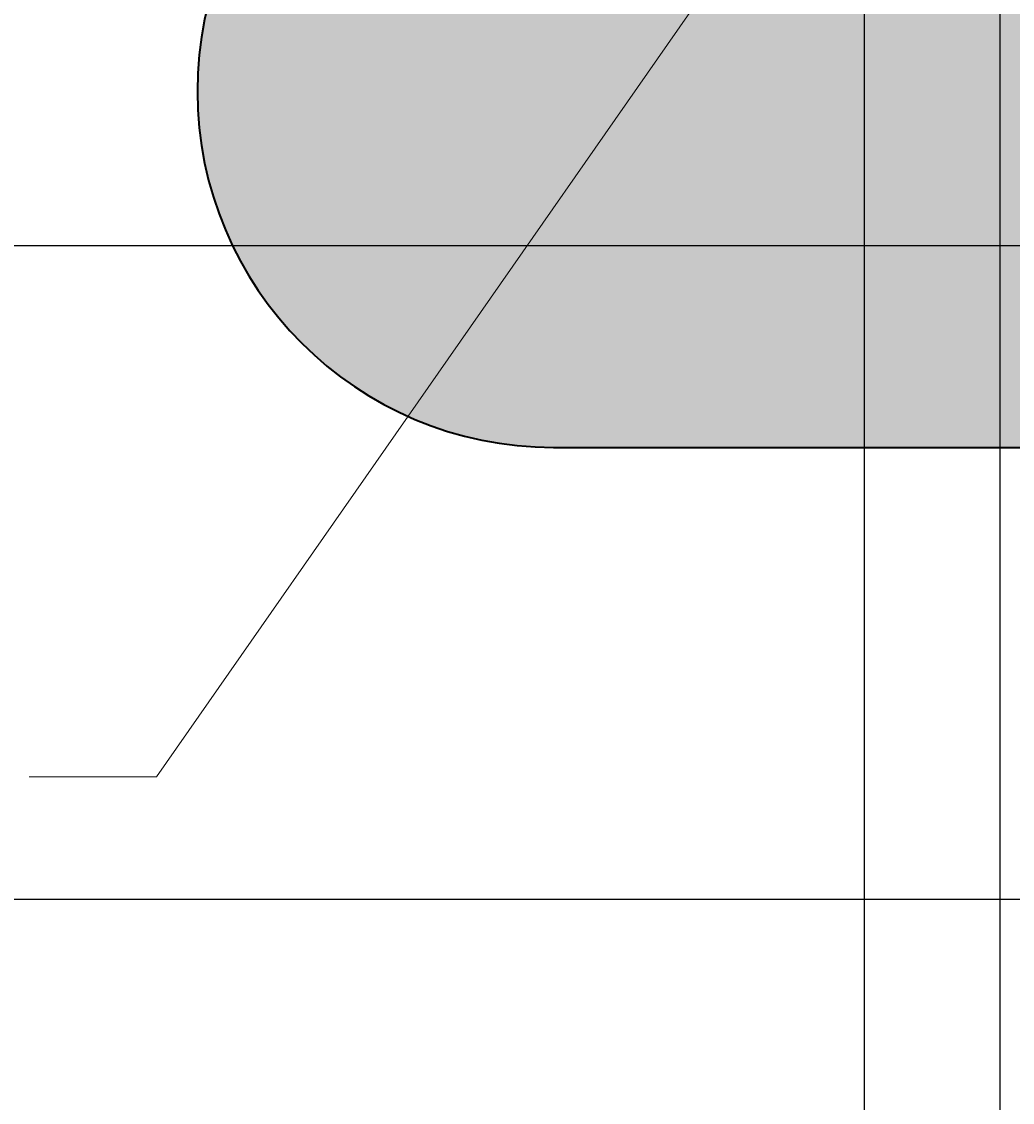
# Model space of a CAD drawing. Units: inches. Extents: x -1 to 292, y -3 to 199.
# Tile 4 of 52: x 46 to 68, y 21 to 45. Entities that reach past the tile are written whole.
import ezdxf

# ---------------------------------------------------------------- set-up
doc = ezdxf.new("R2010")
doc.units = ezdxf.units.IN
doc.header["$MEASUREMENT"] = 0
for name, color, linetype, lineweight in [('M-ANNO-LEAD', 2, 'Continuous', 18), ('M-DIMS', 2, 'Continuous', 18), ('M-EQPM', 7, 'Continuous', 35), ('M-PATT', 8, 'Continuous', 13)]:
    doc.layers.add(name, color=color, linetype=linetype, lineweight=lineweight)
doc.styles.get("Standard").update_dxf_attribs({"font": 'arial.ttf'})
doc.dimstyles.get("Standard").update_dxf_attribs({"dimtxt": 0.18, "dimasz": 0.18, "dimexe": 0.18, "dimexo": 0.0625, "dimgap": 0.09, "dimtad": 0, "dimtih": 1, "dimtoh": 1, "dimdec": 4, "dimzin": 0, "dimdsep": 46, "dimtxsty": 'Standard', "dimcen": 0.09, "dimadec": 0, "dimazin": 0, "dimtfac": 1, "dimtdec": 4, "dimtofl": 0, "dimtmove": 0, "dimatfit": 3, "dimfxl": 1, "dimtolj": 1, "dimtzin": 0, "dimarcsym": 0})

# ---------------------------------------------------------------- blocks, each defined once
blk = doc.blocks.new('*D7')
at = {"layer": 'Defpoints', "color": 0, "transparency": 16777216}
for p in [(21.861, 54.582), (205.115, 54.582), (21.861, 39.982)]:
    blk.add_point(p, dxfattribs=at)
at = {"layer": 'M-DIMS', "color": 0, "lineweight": -2, "transparency": 16777216}
for p, q in [((21.861, 54.52), (21.861, 39.802)), ((205.115, 54.52), (205.115, 39.802)), ((22.041, 39.982), (113.033, 39.982)), ((204.935, 39.982), (113.944, 39.982))]:
    blk.add_line(p, q, dxfattribs=at)
at = {"layer": 'M-DIMS', "color": 0, "transparency": 16777216}
for points in [[(22.041, 40.012), (22.041, 39.952), (21.861, 39.982)], [(204.935, 40.012), (204.935, 39.952), (205.115, 39.982)]]:
    blk.add_solid(points, dxfattribs=at)
at = {"layer": 'M-DIMS', "color": 0, "transparency": 16777216, "insert": (113.488, 39.982), "char_height": 0.18, "attachment_point": 5}
blk.add_mtext('\\A1;183.25', dxfattribs=at)
blk = doc.blocks.new('*D8')
at = {"layer": 'Defpoints', "color": 0, "transparency": 16777216}
for p in [(-0.662, 126.765), (111.488, 126.765), (69.013, 25.514)]:
    blk.add_point(p, dxfattribs=at)
at = {"layer": 'M-DIMS', "color": 0, "lineweight": -2, "transparency": 16777216}
for p, q in [((111.426, 126.765), (-0.842, 126.765)), ((-0.662, 126.585), (-0.662, 76.321)), ((-0.662, 25.694), (-0.662, 75.958)), ((68.951, 25.514), (-0.842, 25.514))]:
    blk.add_line(p, q, dxfattribs=at)
at = {"layer": 'M-DIMS', "color": 0, "transparency": 16777216}
for points in [[(-0.692, 126.585), (-0.632, 126.585), (-0.662, 126.765)], [(-0.692, 25.694), (-0.632, 25.694), (-0.662, 25.514)]]:
    blk.add_solid(points, dxfattribs=at)
at = {"layer": 'M-DIMS', "color": 0, "transparency": 16777216, "insert": (-0.662, 76.14), "char_height": 0.18, "attachment_point": 5}
blk.add_mtext('\\A1;101.25', dxfattribs=at)
blk = doc.blocks.new('*D19')
at = {"layer": 'Defpoints', "color": 0, "transparency": 16777216}
for p in [(64.679, 51.267), (67.679, 51.267), (67.679, -2.71)]:
    blk.add_point(p, dxfattribs=at)
at = {"layer": 'M-DIMS', "color": 0, "lineweight": -2, "transparency": 16777216}
for p, q in [((64.679, 51.205), (64.679, -2.89)), ((67.679, 51.205), (67.679, -2.89)), ((64.859, -2.71), (66.03, -2.71)), ((67.499, -2.71), (66.328, -2.71))]:
    blk.add_line(p, q, dxfattribs=at)
at = {"layer": 'M-DIMS', "color": 0, "transparency": 16777216}
for points in [[(64.859, -2.68), (64.859, -2.74), (64.679, -2.71)], [(67.499, -2.68), (67.499, -2.74), (67.679, -2.71)]]:
    blk.add_solid(points, dxfattribs=at)
at = {"layer": 'M-DIMS', "color": 0, "transparency": 16777216, "insert": (66.179, -2.71), "char_height": 0.18, "attachment_point": 5}
blk.add_mtext('\\A1;3', dxfattribs=at)
blk = doc.blocks.new('*D20')
at = {"layer": 'Defpoints', "color": 0, "transparency": 16777216}
for p in [(64.679, 51.267), (70.679, 51.267), (70.679, -2.71)]:
    blk.add_point(p, dxfattribs=at)
at = {"layer": 'M-DIMS', "color": 0, "lineweight": -2, "transparency": 16777216}
for p, q in [((64.679, 51.205), (64.679, -2.89)), ((70.679, 51.205), (70.679, -2.89)), ((64.859, -2.71), (67.529, -2.71)), ((70.499, -2.71), (67.828, -2.71))]:
    blk.add_line(p, q, dxfattribs=at)
at = {"layer": 'M-DIMS', "color": 0, "transparency": 16777216}
for points in [[(64.859, -2.68), (64.859, -2.74), (64.679, -2.71)], [(70.499, -2.68), (70.499, -2.74), (70.679, -2.71)]]:
    blk.add_solid(points, dxfattribs=at)
at = {"layer": 'M-DIMS', "color": 0, "transparency": 16777216, "insert": (67.679, -2.71), "char_height": 0.18, "attachment_point": 5}
blk.add_mtext('\\A1;6', dxfattribs=at)
blk = doc.blocks.new('*D23')
at = {"layer": 'Defpoints', "color": 0, "transparency": 16777216}
for p in [(21.861, 54.582), (64.679, 51.267), (64.679, -2.71)]:
    blk.add_point(p, dxfattribs=at)
at = {"layer": 'M-DIMS', "color": 0, "lineweight": -2, "transparency": 16777216}
for p, q in [((21.861, 54.52), (21.861, -2.89)), ((64.679, 51.205), (64.679, -2.89)), ((22.041, -2.71), (42.874, -2.71)), ((64.499, -2.71), (43.666, -2.71))]:
    blk.add_line(p, q, dxfattribs=at)
at = {"layer": 'M-DIMS', "color": 0, "transparency": 16777216}
for points in [[(22.041, -2.68), (22.041, -2.74), (21.861, -2.71)], [(64.499, -2.68), (64.499, -2.74), (64.679, -2.71)]]:
    blk.add_solid(points, dxfattribs=at)
at = {"layer": 'M-DIMS', "color": 0, "transparency": 16777216, "insert": (43.27, -2.71), "char_height": 0.18, "attachment_point": 5}
blk.add_mtext('\\A1;42.82', dxfattribs=at)

msp = doc.modelspace()

# ---------------------------------------------------------------- hatches: boundary and pattern name
at = {"layer": 'M-PATT'}
h = msp.add_hatch(color=256, dxfattribs=at)
h.set_gradient(color1=(0, 255, 255), color2=(0, 255, 255), tint=1)
h.paths.add_polyline_path([(75.3521, 99.7735), (72.66, 101.3278), (70.2665, 99.7735), (67.5744, 101.3278), (65.1809, 99.7735), (62.4888, 101.3278), (60.0953, 99.7735), (57.4032, 101.3278), (55.0097, 99.7735), (52.3176, 101.3278), (49.9241, 99.7735, 0.4142136), (57.8007, 91.897), (61.6788, 91.897), (61.6788, 51.2672), (57.8007, 51.2672, 0.8088808), (54.5813, 36.2021), (65.0947, 51.2672), (64.6788, 51.2672), (64.6788, 91.897), (67.6788, 91.897), (67.6788, 51.2672), (65.0947, 51.2672), (54.5813, 36.2021, 0.1056561), (57.8007, 35.5141), (169.176, 35.5141, 1), (169.176, 51.2672), (162.6788, 51.2672), (162.6788, 91.897), (169.176, 91.897, 0.4144629), (177.0526, 99.7802), (174.372, 101.3278), (171.9786, 99.7735), (169.2864, 101.3278), (166.893, 99.7735), (164.2008, 101.3278), (162.1623, 100.004), (162.1623, 96.1027), (160.6222, 96.1027), (160.6222, 100.4578), (159.1152, 101.3278), (156.7218, 99.7735), (154.0296, 101.3278), (151.6362, 99.7735), (148.944, 101.3278), (146.5506, 99.7735), (143.8584, 101.3278), (141.465, 99.7735), (138.7728, 101.3278), (136.3794, 99.7735), (133.6872, 101.3278), (131.2938, 99.7735), (128.6016, 101.3278), (126.2082, 99.7735), (123.516, 101.3278), (121.1225, 99.7735), (118.4304, 101.3278), (116.0369, 99.7735), (113.3448, 101.3278), (110.9513, 99.7735), (108.2592, 101.3278), (105.8657, 99.7735), (103.1736, 101.3278), (100.7801, 99.7735), (98.088, 101.3278), (95.6945, 99.7735), (93.0024, 101.3278), (90.6089, 99.7735), (87.9168, 101.3278), (85.5233, 99.7735), (82.8312, 101.3278), (80.4377, 99.7735), (77.7456, 101.3278)])
h.paths.add_polyline_path([(79.6788, 91.897), (79.6788, 51.2672), (76.6788, 51.2672), (76.6788, 91.897)], flags=16)
h.paths.add_polyline_path([(73.6788, 91.897), (73.6788, 51.2672), (70.6788, 51.2672), (70.6788, 91.897)], flags=16)
h.paths.add_polyline_path([(82.6788, 91.897), (101.6788, 91.897), (101.6788, 51.2672), (82.6788, 51.2672)], flags=16)
h.paths.add_polyline_path([(104.6788, 91.897), (107.6788, 91.897), (107.6788, 51.2672), (104.6788, 51.2672)], flags=16)
h.paths.add_polyline_path([(110.6788, 91.897), (113.6788, 91.897), (113.6788, 51.2672), (110.6788, 51.2672)], flags=16)
h.paths.add_polyline_path([(116.6788, 91.897), (119.6788, 91.897), (119.6788, 51.2672), (116.6788, 51.2672)], flags=16)
h.paths.add_polyline_path([(122.6788, 91.897), (141.6788, 91.897), (141.6788, 51.2672), (144.6788, 51.2672), (144.6788, 91.897), (147.6788, 91.897), (147.6788, 51.2672), (122.6788, 51.2672)], flags=16)
h.paths.add_polyline_path([(150.6788, 91.897), (153.6788, 91.897), (153.6788, 51.2672), (150.6788, 51.2672)], flags=16)
h.paths.add_polyline_path([(156.6788, 91.897), (159.6788, 91.897), (159.6788, 51.2672), (156.6788, 51.2672)], flags=16)

# ---------------------------------------------------------------- linework, layer by layer
at = {"layer": 'M-ANNO-LEAD'}
for p, q in [((66.2726, 52.955), (49.017, 28.2287)), ((49.017, 28.2287), (46.2035, 28.2287))]:
    msp.add_line(p, q, dxfattribs=at)
at = {"layer": 'M-EQPM'}
msp.add_lwpolyline([(61.6788, 51.2672), (57.8007, 51.2672, 1), (57.8007, 35.5141), (169.176, 35.5141, 1), (169.176, 51.2672), (162.6788, 51.2672)], format="xyb", dxfattribs=at)

# ---------------------------------------------------------------- dimensions: what is measured, and where the dimension line sits
at = {"layer": 'M-DIMS'}
for base, p1, p2, angle, picture, middle in [((-0.6625, 126.765), (69.013, 25.5141), (111.4883, 126.765), 90, '*D8', (-0.6625, 76.1396)), ((21.8612, 39.9821), (205.1155, 54.5821), (21.8612, 54.5821), 180, '*D7', (113.4883, 39.9821))]:
    dim = msp.add_linear_dim(base=base, p1=p1, p2=p2, angle=angle, dimstyle='Standard', override={"dimdec": 2, "dimlfac": 1, "dimrnd": 0, "dimzin": 0, "dimdsep": 46, "dimlunit": 2}, dxfattribs=at)
    dim.commit()
    dim.dimension.update_dxf_attribs({"geometry": picture, "text_midpoint": middle})
for base, p1, p2, override, picture, middle in [((64.6788, -2.7104), (21.8612, 54.5821), (64.6788, 51.2672), {"dimdec": 2, "dimlfac": 1, "dimrnd": 0, "dimzin": 0, "dimdsep": 46, "dimlunit": 2}, '*D23', (43.27, -2.7104)), ((67.6788, -2.7104), (64.6788, 51.2672), (67.6788, 51.2672), {"dimdec": 0, "dimlfac": 1, "dimrnd": 0, "dimzin": 0, "dimdsep": 46, "dimlunit": 2}, '*D19', (66.1788, -2.7104)), ((70.6788, -2.7104), (64.6788, 51.2672), (70.6788, 51.2672), {"dimdec": 0, "dimlfac": 1, "dimrnd": 0, "dimzin": 0, "dimdsep": 46, "dimlunit": 2}, '*D20', (67.6788, -2.7104))]:
    dim = msp.add_linear_dim(base=base, p1=p1, p2=p2, dimstyle='Standard', override=override, dxfattribs=at)
    dim.commit()
    dim.dimension.update_dxf_attribs({"geometry": picture, "text_midpoint": middle})

doc.saveas('drawing.dxf')
